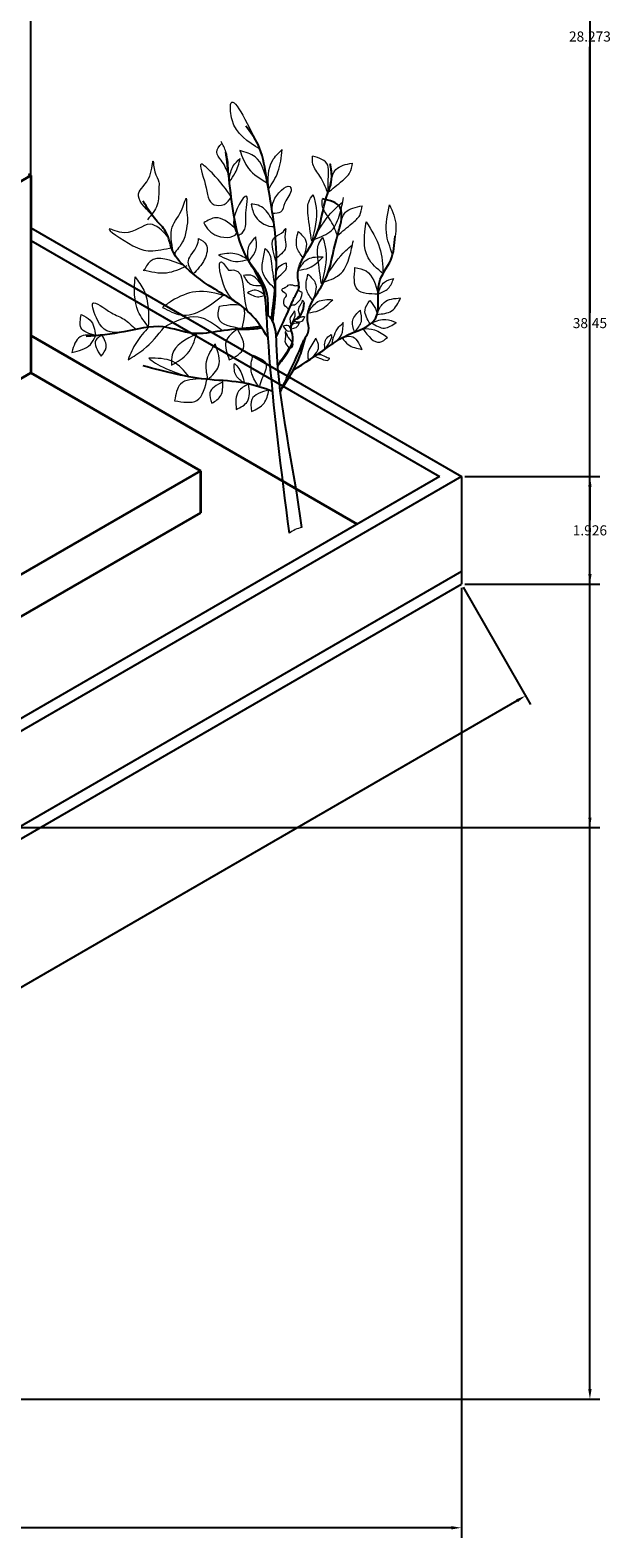
# Model space of a CAD drawing. Units: metres. Extents: x 12735 to 25554, y 20954 to 41989.
# Tile 14 of 15: x 12773 to 12784, y 20954 to 20981. Entities that reach past the tile are written whole.
import ezdxf

# ---------------------------------------------------------------- set-up
doc = ezdxf.new("R2010")
doc.units = ezdxf.units.M
doc.layers.get('Defpoints').update_dxf_attribs({"lineweight": 13})
for name, color, linetype, lineweight in [('A-ANNO-DIMS', 2, 'Continuous', 18), ('A-ELEV', 7, 'Continuous', 35), ('C-SITE', 8, 'Continuous', 25), ('TREES', 72, 'Continuous', 18)]:
    doc.layers.add(name, color=color, linetype=linetype, lineweight=lineweight)
doc.layers.add('STEM', color=32, linetype='Continuous')
doc.styles.get("Standard").update_dxf_attribs({"font": 'arial.ttf'})
doc.dimstyles.get("Standard").update_dxf_attribs({"dimtxt": 0.18, "dimasz": 0.18, "dimexe": 0.18, "dimexo": 0.0625, "dimgap": 0.09, "dimtad": 0, "dimtih": 1, "dimtoh": 1, "dimdec": 4, "dimzin": 0, "dimdsep": 46, "dimtxsty": 'Standard', "dimcen": 0.09, "dimadec": 0, "dimazin": 0, "dimtfac": 1, "dimtdec": 4, "dimtofl": 0, "dimtmove": 0, "dimatfit": 3, "dimfxl": 1, "dimtolj": 1, "dimtzin": 0, "dimarcsym": 0})

# ---------------------------------------------------------------- blocks, each defined once
blk = doc.blocks.new('TREES')
blk.add_line((12743.7, 20972.648), (12743.7, 20972.648))
at = {"layer": 'STEM'}
for points, knots in [([(12743.791, 20972.546), (12743.793, 20972.564), (12743.795, 20972.582), (12743.797, 20972.6), (12743.801, 20972.637), (12743.806, 20972.674), (12743.81, 20972.711), (12743.845, 20973.018), (12743.938, 20973.826), (12743.743, 20974.806), (12743.607, 20975.634), (12743.413, 20975.893), (12743.333, 20975.999)], [-0.164913, -0.164913, -0.164913, -0.164913, -0.110972, -0.110972, -0.110972, 0, 0, 0, 0.920963, 2.426088, 2.990404, 3.384799, 3.384799, 3.384799, 3.384799]), ([(12743.7, 20972.648), (12743.691, 20972.807), (12743.671, 20973.194), (12743.257, 20973.699), (12743.111, 20974.379), (12743.038, 20974.998), (12742.993, 20975.377), (12742.974, 20975.54)], [0, 0, 0, 0, 0.469346, 1.137622, 1.869488, 2.521439, 3.013071, 3.013071, 3.013071, 3.013071]), ([(12743.874, 20972.227), (12743.898, 20972.277), (12743.921, 20972.328), (12743.945, 20972.378), (12744.022, 20972.541), (12744.105, 20972.717), (12744.205, 20972.963), (12744.312, 20973.088), (12744.183, 20973.501), (12744.667, 20973.973), (12744.707, 20974.64), (12744.896, 20975.012), (12744.823, 20975.434), (12744.85, 20975.23), (12744.867, 20975.1)], [-0.166951, -0.166951, -0.166951, -0.166951, 0, 0, 0, 0.539768, 0.582066, 0.798222, 0.98781, 1.7696, 2.524754, 2.899414, 3.105113, 3.460848, 3.460848, 3.460848, 3.460848]), ([(12743.728, 20972.218), (12743.63, 20972.372), (12743.383, 20972.76), (12742.753, 20973.07), (12742.291, 20973.419), (12741.984, 20973.759), (12741.959, 20974.098), (12741.675, 20974.346), (12741.563, 20974.543), (12741.494, 20974.663)], [0, 0, 0, 0, 0.542161, 1.359078, 2.03444, 2.290187, 2.703676, 2.968549, 3.382864, 3.382864, 3.382864, 3.382864]), ([(12743.967, 20971.294), (12743.987, 20971.335), (12744.006, 20971.376), (12744.026, 20971.417), (12744.057, 20971.483), (12744.088, 20971.549), (12744.119, 20971.615), (12744.196, 20971.778), (12744.279, 20971.954), (12744.378, 20972.2), (12744.486, 20972.325), (12744.357, 20972.738), (12744.836, 20973.215), (12744.895, 20973.862), (12745.051, 20974.269), (12745.045, 20974.62), (12744.834, 20974.67), (12744.7, 20974.701)], [-0.355099, -0.355099, -0.355099, -0.355099, -0.218492, -0.218492, -0.218492, 0, 0, 0, 0.539768, 0.582066, 0.798222, 0.98781, 1.7696, 2.524754, 2.899414, 3.105113, 3.460848, 3.460848, 3.460848, 3.460848]), ([(12744.175, 20971.633), (12744.383, 20971.767), (12744.692, 20971.967), (12745.149, 20972.305), (12745.828, 20972.463), (12745.606, 20973.185), (12745.967, 20973.583), (12745.99, 20973.882), (12746.002, 20974.029)], [0, 0, 0, 0, 0.736164, 1.094646, 1.754618, 2.392389, 2.840214, 3.27091, 3.27091, 3.27091, 3.27091]), ([(12743.381, 20973.588), (12743.52, 20973.4), (12743.728, 20973.118), (12743.725, 20972.776), (12743.724, 20972.661), (12743.724, 20972.661), (12743.724, 20972.661), (12743.724, 20972.661), (12743.724, 20972.65), (12743.724, 20972.639), (12743.724, 20972.627)], [0, 0, 0, 0, 0.673099, 1.009429, 1.009429, 1.009429, 1.009429, 1.009429, 1.009429, 1.043412, 1.043412, 1.043412, 1.043412]), ([(12743.814, 20972.505), (12743.817, 20972.531), (12743.819, 20972.556), (12743.822, 20972.581), (12743.827, 20972.63), (12743.832, 20972.679), (12743.838, 20972.727), (12743.847, 20972.813), (12743.865, 20972.982), (12743.864, 20973.152), (12743.864, 20973.236)], [-0.2227932, -0.2227932, -0.2227932, -0.2227932, -0.1464713, -0.1464713, -0.1464713, 0, 0, 0, 0.2578951, 0.5103882, 0.5103882, 0.5103882, 0.5103882]), ([(12743.902, 20971.717), (12743.93, 20971.754), (12743.959, 20971.791), (12743.988, 20971.829), (12743.988, 20971.829), (12743.988, 20971.829), (12743.988, 20971.829), (12744.096, 20971.973), (12744.236, 20972.16), (12744.082, 20972.476), (12744.347, 20972.598), (12744.368, 20972.766), (12744.376, 20972.837)], [-0.129757, -0.129757, -0.129757, -0.129757, 0, 0, 0, 0, 0, 0, 0.485118, 0.62751, 0.913144, 1.120766, 1.120766, 1.120766, 1.120766]), ([(12744.111, 20968.725), (12743.967, 20969.837), (12743.799, 20971.142), (12743.712, 20972.453), (12743.7, 20972.648)], [0, 0, 0, 0, 3.359203, 3.944548, 3.944548, 3.944548, 3.944548]), ([(12744.332, 20968.825), (12744.189, 20969.936), (12743.871, 20971.161), (12743.872, 20972.51), (12743.7, 20972.648)], [0, 0, 0, 0, 3.359203, 3.972384, 3.972384, 3.972384, 3.972384]), ([(12743.597, 20972.418), (12743.533, 20972.41), (12743.292, 20972.379), (12742.889, 20972.351), (12742.364, 20972.241), (12741.803, 20972.489), (12741.157, 20972.302), (12740.698, 20972.258), (12740.474, 20972.237)], [0, 0, 0, 0, 0.193148, 0.727923, 1.218416, 1.762371, 2.471743, 3.152626, 3.152626, 3.152626, 3.152626]), ([(12743.181, 20972.372), (12743.296, 20972.37), (12743.441, 20972.368), (12743.583, 20972.39), (12743.613, 20972.395)], [0, 0, 0, 0, 0.3435042, 0.4329772, 0.4329772, 0.4329772, 0.4329772]), ([(12743.948, 20971.264), (12743.975, 20971.305), (12744.002, 20971.345), (12744.029, 20971.386), (12744.029, 20971.386), (12744.029, 20971.386), (12744.029, 20971.386), (12744.129, 20971.55), (12744.289, 20971.812), (12744.368, 20972.107), (12744.398, 20972.218)], [-0.148605, -0.148605, -0.148605, -0.148605, 0, 0, 0, 0, 0, 0, 0.572176, 0.914425, 0.914425, 0.914425, 0.914425]), ([(12743.901, 20971.729), (12743.929, 20971.768), (12743.958, 20971.808), (12743.986, 20971.847), (12743.986, 20971.847), (12743.986, 20971.847), (12743.986, 20971.847), (12744.02, 20971.892), (12744.062, 20971.951), (12744.099, 20972.014), (12744.107, 20972.028)], [-0.1467707, -0.1467707, -0.1467707, -0.1467707, 0, 0, 0, 0, 0, 0, 0.1684242, 0.2179474, 0.2179474, 0.2179474, 0.2179474]), ([(12743.81, 20971.258), (12743.646, 20971.316), (12743.283, 20971.443), (12742.486, 20971.453), (12741.888, 20971.61), (12741.494, 20971.714)], [0, 0, 0, 0, 0.519056, 1.146346, 2.366016, 2.366016, 2.366016, 2.366016])]:
    blk.add_open_spline(points, degree=3, knots=knots, dxfattribs=at)
blk.add_open_spline([(12744.644, 20971.941), (12744.672, 20971.961), (12744.701, 20971.98), (12744.73, 20972)], degree=3, dxfattribs=at)
at = {"layer": 'TREES'}
for points, knots in [([(12743.584, 20975.586), (12743.37, 20975.718), (12743.075, 20975.9), (12743.022, 20976.725), (12743.333, 20976.097), (12743.574, 20975.612)], [0, 0, 0, 0, 0.724771, 1.002271, 1.932196, 1.932196, 1.932196, 1.932196]), ([(12743.021, 20975.14), (12742.985, 20975.224), (12742.928, 20975.356), (12742.766, 20975.539), (12742.854, 20975.638), (12742.901, 20975.69)], [0, 0, 0, 0, 0.2845416, 0.4465287, 0.6279758, 0.6279758, 0.6279758, 0.6279758]), ([(12743.021, 20975.14), (12743.019, 20975.277), (12743.016, 20975.483), (12742.921, 20975.662), (12742.889, 20975.721)], [0, 0, 0, 0, 0.4023849, 0.6031293, 0.6031293, 0.6031293, 0.6031293]), ([(12743.031, 20975.058), (12743.048, 20975.139), (12743.077, 20975.281), (12743.184, 20975.377), (12743.231, 20975.418)], [0, 0, 0, 0, 0.2398723, 0.4207027, 0.4207027, 0.4207027, 0.4207027]), ([(12743.037, 20975.007), (12743.075, 20975.058), (12743.166, 20975.181), (12743.207, 20975.33), (12743.231, 20975.418)], [0, 0, 0, 0, 0.1895117, 0.457602, 0.457602, 0.457602, 0.457602]), ([(12743.718, 20974.979), (12743.671, 20975.164), (12743.598, 20975.454), (12743.323, 20975.534), (12743.223, 20975.563)], [0, 0, 0, 0, 0.519429, 0.8155501, 0.8155501, 0.8155501, 0.8155501]), ([(12743.223, 20975.563), (12743.266, 20975.448), (12743.36, 20975.195), (12743.592, 20975.055), (12743.718, 20974.979)], [0, 0, 0, 0, 0.3595778, 0.7860105, 0.7860105, 0.7860105, 0.7860105]), ([(12743.737, 20974.871), (12743.729, 20975.055), (12743.718, 20975.333), (12743.914, 20975.516), (12743.981, 20975.578)], [0, 0, 0, 0, 0.5134638, 0.7779111, 0.7779111, 0.7779111, 0.7779111]), ([(12743.737, 20974.871), (12743.801, 20974.971), (12743.939, 20975.186), (12743.966, 20975.441), (12743.981, 20975.578)], [0, 0, 0, 0, 0.351068, 0.7565079, 0.7565079, 0.7565079, 0.7565079]), ([(12744.796, 20974.806), (12744.757, 20974.909), (12744.688, 20975.088), (12744.514, 20975.28), (12744.523, 20975.414), (12744.526, 20975.464)], [0, 0, 0, 0, 0.3323117, 0.5782809, 0.7232611, 0.7232611, 0.7232611, 0.7232611]), ([(12744.805, 20974.813), (12744.804, 20974.918), (12744.803, 20975.076), (12744.822, 20975.37), (12744.643, 20975.427), (12744.526, 20975.464)], [0, 0, 0, 0, 0.3224266, 0.4885617, 0.8037384, 0.8037384, 0.8037384, 0.8037384]), ([(12741.648, 20974.411), (12741.519, 20974.547), (12741.281, 20974.798), (12741.642, 20974.995), (12741.673, 20975.511), (12741.684, 20975.149), (12741.787, 20975.033), (12741.768, 20974.824), (12741.781, 20974.575), (12741.641, 20974.411), (12741.569, 20974.326)], [0, 0, 0, 0, 0.446457, 0.821839, 1.096823, 1.294203, 1.491123, 1.594729, 1.894892, 2.216107, 2.216107, 2.216107, 2.216107]), ([(12743.07, 20974.733), (12742.98, 20974.863), (12742.848, 20975.053), (12742.433, 20975.446), (12742.649, 20974.915), (12742.651, 20974.573), (12742.961, 20974.576), (12743.034, 20974.678), (12743.071, 20974.73)], [0, 0, 0, 0, 0.54832, 0.799685, 1.166614, 1.565159, 1.742127, 1.925713, 1.925713, 1.925713, 1.925713]), ([(12744.796, 20974.806), (12744.882, 20974.878), (12745.017, 20974.992), (12745.211, 20975.15), (12745.228, 20975.277), (12745.236, 20975.337)], [0, 0, 0, 0, 0.3416822, 0.5370609, 0.7122352, 0.7122352, 0.7122352, 0.7122352]), ([(12744.839, 20974.951), (12744.859, 20975.055), (12744.903, 20975.272), (12745.122, 20975.315), (12745.236, 20975.337)], [0, 0, 0, 0, 0.2913456, 0.6064398, 0.6064398, 0.6064398, 0.6064398]), ([(12743.814, 20974.4), (12743.798, 20974.494), (12743.764, 20974.693), (12744.115, 20975.006), (12744.156, 20974.79), (12744.01, 20974.677), (12743.989, 20974.434), (12743.864, 20974.438), (12743.809, 20974.439)], [0, 0, 0, 0, 0.311146, 0.650746, 0.669061, 0.940573, 1.125337, 1.270427, 1.270427, 1.270427, 1.270427]), ([(12742.028, 20973.754), (12742.003, 20973.912), (12741.953, 20974.218), (12742.174, 20974.414), (12742.283, 20974.81), (12742.258, 20974.48), (12742.304, 20974.323), (12742.246, 20974.069), (12742.227, 20973.932), (12742.006, 20973.671), (12742.066, 20973.72), (12742.075, 20973.727)], [0, 0, 0, 0, 0.436736, 0.842969, 1.012738, 1.21393, 1.403734, 1.613178, 1.897283, 2.067562, 2.097274, 2.097274, 2.097274, 2.097274]), ([(12743.191, 20974.047), (12743.14, 20974.139), (12743.026, 20974.346), (12743.367, 20974.877), (12743.354, 20974.597), (12743.309, 20974.413), (12743.358, 20974.125), (12743.218, 20974.059), (12743.191, 20974.047)], [0, 0, 0, 0, 0.337622, 0.758697, 0.837919, 1.040495, 1.406258, 1.489574, 1.489574, 1.489574, 1.489574]), ([(12744.509, 20973.941), (12744.486, 20974.093), (12744.451, 20974.322), (12744.425, 20974.623), (12744.504, 20974.731), (12744.534, 20974.773)], [0, 0, 0, 0, 0.4681587, 0.7056034, 0.8580265, 0.8580265, 0.8580265, 0.8580265]), ([(12744.534, 20974.773), (12744.556, 20974.698), (12744.634, 20974.425), (12744.562, 20974.144), (12744.509, 20973.941)], [0, 0, 0, 0, 0.2327329, 0.8431329, 0.8431329, 0.8431329, 0.8431329]), ([(12744.554, 20973.975), (12744.669, 20974.016), (12744.893, 20974.094), (12745.019, 20974.421), (12745.06, 20974.624), (12745.08, 20974.72)], [0, 0, 0, 0, 0.348929, 0.678298, 0.9763146, 0.9763146, 0.9763146, 0.9763146]), ([(12744.618, 20974.118), (12744.717, 20974.268), (12744.844, 20974.462), (12745.022, 20974.606), (12745.062, 20974.638)], [0, 0, 0, 0, 0.5333846, 0.686651, 0.686651, 0.686651, 0.686651]), ([(12744.97, 20974.043), (12744.931, 20974.146), (12744.862, 20974.325), (12744.688, 20974.517), (12744.697, 20974.651), (12744.7, 20974.701)], [0, 0, 0, 0, 0.3323117, 0.5782809, 0.7232611, 0.7232611, 0.7232611, 0.7232611]), ([(12743.128, 20974.182), (12743.019, 20974.275), (12742.841, 20974.427), (12742.65, 20974.313), (12742.577, 20974.27)], [0, 0, 0, 0, 0.3785086, 0.6144536, 0.6144536, 0.6144536, 0.6144536]), ([(12743.835, 20974.249), (12743.789, 20974.346), (12743.724, 20974.484), (12743.556, 20974.594), (12743.468, 20974.601), (12743.424, 20974.604)], [0, 0, 0, 0, 0.3158223, 0.4463774, 0.5774617, 0.5774617, 0.5774617, 0.5774617]), ([(12743.424, 20974.604), (12743.442, 20974.527), (12743.487, 20974.324), (12743.715, 20974.191), (12743.841, 20974.206), (12743.841, 20974.206)], [0, 0, 0, 0, 0.2361186, 0.6165307, 0.6167763, 0.6167763, 0.6167763, 0.6167763]), ([(12744.97, 20974.043), (12745.056, 20974.115), (12745.191, 20974.229), (12745.385, 20974.387), (12745.402, 20974.514), (12745.41, 20974.574)], [0, 0, 0, 0, 0.3416822, 0.5370609, 0.7122352, 0.7122352, 0.7122352, 0.7122352]), ([(12745.013, 20974.188), (12745.033, 20974.292), (12745.077, 20974.509), (12745.296, 20974.552), (12745.41, 20974.574)], [0, 0, 0, 0, 0.2913456, 0.6064398, 0.6064398, 0.6064398, 0.6064398]), ([(12745.957, 20973.706), (12745.908, 20973.835), (12745.798, 20974.123), (12745.864, 20974.427), (12745.9, 20974.594)], [0, 0, 0, 0, 0.4051126, 0.906838, 0.906838, 0.906838, 0.906838]), ([(12745.9, 20974.594), (12745.955, 20974.471), (12746.037, 20974.287), (12746.01, 20974.092), (12746.002, 20974.029)], [0, 0, 0, 0, 0.3943838, 0.5836156, 0.5836156, 0.5836156, 0.5836156]), ([(12741.943, 20974.016), (12741.835, 20974.13), (12741.594, 20974.382), (12741.272, 20973.991), (12740.687, 20974.27), (12741.289, 20973.836), (12741.63, 20973.742), (12741.878, 20973.799), (12742.016, 20973.831)], [0, 0, 0, 0, 0.397812, 0.88569, 1.156328, 1.66735, 1.991498, 2.394837, 2.394837, 2.394837, 2.394837]), ([(12742.577, 20974.27), (12742.635, 20974.174), (12742.755, 20973.977), (12743.187, 20974.003), (12743.173, 20974.131), (12743.172, 20974.137)], [0, 0, 0, 0, 0.3386751, 0.6999446, 0.7185805, 0.7185805, 0.7185805, 0.7185805]), ([(12743.879, 20973.555), (12743.816, 20973.752), (12743.731, 20974.021), (12743.982, 20974.067), (12744.068, 20974.224), (12744.006, 20973.984), (12744.093, 20973.824), (12743.961, 20973.709), (12743.879, 20973.638)], [0, 0, 0, 0, 0.469961, 0.638827, 0.705595, 0.853148, 1.022788, 1.296962, 1.296962, 1.296962, 1.296962]), ([(12744.356, 20973.647), (12744.309, 20973.708), (12744.202, 20973.846), (12744.245, 20974.018), (12744.268, 20974.113)], [0, 0, 0, 0, 0.2209277, 0.4981889, 0.4981889, 0.4981889, 0.4981889]), ([(12744.268, 20974.113), (12744.323, 20974.065), (12744.46, 20973.94), (12744.395, 20973.758), (12744.356, 20973.647)], [0, 0, 0, 0, 0.203616, 0.5174389, 0.5174389, 0.5174389, 0.5174389]), ([(12745.785, 20973.361), (12745.68, 20973.449), (12745.404, 20973.684), (12745.451, 20974.057), (12745.481, 20974.288)], [0, 0, 0, 0, 0.391493, 1.034106, 1.034106, 1.034106, 1.034106]), ([(12745.481, 20974.288), (12745.577, 20974.138), (12745.76, 20973.855), (12745.777, 20973.519), (12745.785, 20973.361)], [0, 0, 0, 0, 0.5245256, 0.9915723, 0.9915723, 0.9915723, 0.9915723]), ([(12742.389, 20973.356), (12742.341, 20973.437), (12742.234, 20973.617), (12742.458, 20973.799), (12742.48, 20973.946), (12742.486, 20973.991)], [0, 0, 0, 0, 0.251735, 0.5591808, 0.6938707, 0.6938707, 0.6938707, 0.6938707]), ([(12742.486, 20973.991), (12742.542, 20973.959), (12742.68, 20973.88), (12742.598, 20973.572), (12742.464, 20973.433), (12742.389, 20973.356)], [0, 0, 0, 0, 0.1746142, 0.4385715, 0.7703441, 0.7703441, 0.7703441, 0.7703441]), ([(12743.381, 20973.588), (12743.369, 20973.67), (12743.344, 20973.833), (12743.453, 20973.958), (12743.508, 20974.02)], [0, 0, 0, 0, 0.2360196, 0.4713289, 0.4713289, 0.4713289, 0.4713289]), ([(12743.381, 20973.588), (12743.434, 20973.649), (12743.541, 20973.774), (12743.519, 20973.937), (12743.508, 20974.02)], [0, 0, 0, 0, 0.2309694, 0.4699481, 0.4699481, 0.4699481, 0.4699481]), ([(12743.851, 20973.09), (12743.747, 20973.196), (12743.578, 20973.368), (12743.647, 20973.644), (12743.671, 20973.769), (12743.679, 20973.81)], [0, 0, 0, 0, 0.4076044, 0.6640272, 0.7921335, 0.7921335, 0.7921335, 0.7921335]), ([(12743.679, 20973.81), (12743.708, 20973.778), (12743.776, 20973.703), (12743.798, 20973.443), (12743.829, 20973.238), (12743.851, 20973.09)], [0, 0, 0, 0, 0.125659, 0.2981213, 0.7527794, 0.7527794, 0.7527794, 0.7527794]), ([(12744.683, 20973.178), (12744.66, 20973.33), (12744.625, 20973.559), (12744.599, 20973.86), (12744.677, 20973.968), (12744.708, 20974.01)], [0, 0, 0, 0, 0.4681587, 0.7056034, 0.8580265, 0.8580265, 0.8580265, 0.8580265]), ([(12744.708, 20974.01), (12744.73, 20973.935), (12744.807, 20973.662), (12744.735, 20973.381), (12744.683, 20973.178)], [0, 0, 0, 0, 0.2327329, 0.8431329, 0.8431329, 0.8431329, 0.8431329]), ([(12744.728, 20973.213), (12744.843, 20973.253), (12745.067, 20973.331), (12745.193, 20973.658), (12745.234, 20973.861), (12745.254, 20973.957)], [0, 0, 0, 0, 0.348929, 0.678298, 0.9763146, 0.9763146, 0.9763146, 0.9763146]), ([(12744.792, 20973.355), (12744.891, 20973.505), (12745.018, 20973.699), (12745.196, 20973.843), (12745.236, 20973.876)], [0, 0, 0, 0, 0.5333846, 0.686651, 0.686651, 0.686651, 0.686651]), ([(12742.221, 20973.506), (12741.989, 20973.602), (12741.674, 20973.731), (12741.536, 20973.471), (12741.5, 20973.404)], [0, 0, 0, 0, 0.6060397, 0.8197481, 0.8197481, 0.8197481, 0.8197481]), ([(12743.253, 20972.784), (12743.147, 20972.854), (12742.919, 20973.005), (12742.8, 20973.728), (12742.973, 20973.491), (12743.022, 20973.422)], [0, 0, 0, 0, 0.420416, 0.90702, 1.103207, 1.103207, 1.103207, 1.103207]), ([(12743.364, 20973.617), (12743.288, 20973.661), (12743.124, 20973.754), (12742.939, 20973.715), (12742.84, 20973.694)], [0, 0, 0, 0, 0.2535199, 0.5460217, 0.5460217, 0.5460217, 0.5460217]), ([(12742.84, 20973.694), (12742.956, 20973.634), (12743.128, 20973.545), (12743.306, 20973.6), (12743.364, 20973.617)], [0, 0, 0, 0, 0.369417, 0.546183, 0.546183, 0.546183, 0.546183]), ([(12743.864, 20973.236), (12743.891, 20973.272), (12743.952, 20973.35), (12744.077, 20973.438), (12744.058, 20973.527), (12744.051, 20973.558)], [0, 0, 0, 0, 0.1377377, 0.3031534, 0.3935537, 0.3935537, 0.3935537, 0.3935537]), ([(12743.866, 20973.267), (12743.872, 20973.352), (12743.881, 20973.49), (12744.004, 20973.539), (12744.051, 20973.558)], [0, 0, 0, 0, 0.2295676, 0.3730638, 0.3730638, 0.3730638, 0.3730638]), ([(12744.268, 20973.425), (12744.32, 20973.505), (12744.424, 20973.666), (12744.615, 20973.662), (12744.711, 20973.66)], [0, 0, 0, 0, 0.2669279, 0.5349854, 0.5349854, 0.5349854, 0.5349854]), ([(12744.268, 20973.425), (12744.336, 20973.433), (12744.51, 20973.454), (12744.635, 20973.582), (12744.711, 20973.66)], [0, 0, 0, 0, 0.1990667, 0.5143408, 0.5143408, 0.5143408, 0.5143408]), ([(12741.595, 20972.406), (12741.523, 20972.496), (12741.318, 20972.752), (12741.336, 20973.087), (12741.348, 20973.304)], [0, 0, 0, 0, 0.3390919, 0.9589007, 0.9589007, 0.9589007, 0.9589007]), ([(12741.348, 20973.304), (12741.406, 20973.227), (12741.6, 20972.969), (12741.591, 20972.637), (12741.585, 20972.405)], [0, 0, 0, 0, 0.2865181, 0.9509807, 0.9509807, 0.9509807, 0.9509807]), ([(12741.493, 20973.429), (12741.634, 20973.396), (12741.906, 20973.333), (12742.16, 20973.449), (12742.283, 20973.505)], [0, 0, 0, 0, 0.420024, 0.8136231, 0.8136231, 0.8136231, 0.8136231]), ([(12743.022, 20973.422), (12743.059, 20973.426), (12743.334, 20973.456), (12743.256, 20972.956), (12743.349, 20972.723), (12743.36, 20972.696)], [0, 0, 0, 0, 0.1039343, 0.7792863, 0.8705393, 0.8705393, 0.8705393, 0.8705393]), ([(12743.621, 20973.151), (12743.561, 20973.233), (12743.473, 20973.354), (12743.333, 20973.334), (12743.288, 20973.327)], [0, 0, 0, 0, 0.2726158, 0.4022356, 0.4022356, 0.4022356, 0.4022356]), ([(12743.288, 20973.327), (12743.325, 20973.265), (12743.399, 20973.138), (12743.546, 20973.147), (12743.621, 20973.151)], [0, 0, 0, 0, 0.199886, 0.4070645, 0.4070645, 0.4070645, 0.4070645]), ([(12744.53, 20972.884), (12744.482, 20972.945), (12744.376, 20973.084), (12744.419, 20973.255), (12744.442, 20973.351)], [0, 0, 0, 0, 0.2209277, 0.4981889, 0.4981889, 0.4981889, 0.4981889]), ([(12744.442, 20973.351), (12744.496, 20973.302), (12744.634, 20973.177), (12744.569, 20972.995), (12744.53, 20972.884)], [0, 0, 0, 0, 0.203616, 0.5174389, 0.5174389, 0.5174389, 0.5174389]), ([(12745.697, 20972.996), (12745.547, 20972.999), (12745.238, 20973.004), (12745.268, 20973.314), (12745.283, 20973.473)], [0, 0, 0, 0, 0.3799868, 0.779071, 0.779071, 0.779071, 0.779071]), ([(12745.283, 20973.473), (12745.354, 20973.458), (12745.585, 20973.409), (12745.651, 20973.165), (12745.697, 20972.996)], [0, 0, 0, 0, 0.2074949, 0.6743984, 0.6743984, 0.6743984, 0.6743984]), ([(12745.697, 20972.996), (12745.724, 20973.08), (12745.77, 20973.226), (12745.915, 20973.262), (12745.976, 20973.277)], [0, 0, 0, 0, 0.2439478, 0.4222058, 0.4222058, 0.4222058, 0.4222058]), ([(12745.697, 20972.996), (12745.764, 20973.024), (12745.897, 20973.078), (12745.95, 20973.211), (12745.976, 20973.277)], [0, 0, 0, 0, 0.2073861, 0.4117039, 0.4117039, 0.4117039, 0.4117039]), ([(12742.983, 20972.961), (12742.799, 20973.009), (12742.463, 20973.098), (12742.071, 20972.928), (12741.893, 20972.798), (12741.839, 20972.759)], [0, 0, 0, 0, 0.553894, 1.01265, 1.215779, 1.215779, 1.215779, 1.215779]), ([(12743.669, 20972.977), (12743.606, 20973.025), (12743.504, 20973.102), (12743.398, 20973.043), (12743.358, 20973.021)], [0, 0, 0, 0, 0.2119595, 0.340544, 0.340544, 0.340544, 0.340544]), ([(12743.358, 20973.021), (12743.426, 20972.983), (12743.527, 20972.926), (12743.633, 20972.964), (12743.669, 20972.977)], [0, 0, 0, 0, 0.2166399, 0.3265492, 0.3265492, 0.3265492, 0.3265492]), ([(12744.074, 20972.655), (12744.086, 20972.673), (12744.124, 20972.731), (12743.998, 20972.782), (12744.014, 20972.867), (12744.011, 20972.925), (12744.052, 20972.944), (12744.07, 20973.015), (12743.988, 20973.027), (12743.97, 20973.091), (12744.03, 20973.11), (12744.072, 20973.132), (12744.097, 20973.169), (12744.133, 20973.163), (12744.172, 20973.164), (12744.216, 20973.136), (12744.296, 20973.17), (12744.282, 20973.105), (12744.259, 20973.057), (12744.341, 20973.048), (12744.328, 20972.986), (12744.32, 20972.935), (12744.299, 20972.884), (12744.258, 20972.852), (12744.236, 20972.821), (12744.215, 20972.805), (12744.179, 20972.793), (12744.139, 20972.807), (12744.095, 20972.746), (12744.111, 20972.739), (12744.111, 20972.739)], [0, 0, 0, 0, 0.055886, 0.185472, 0.25227, 0.305988, 0.338368, 0.378405, 0.48523, 0.4997, 0.565031, 0.618654, 0.656012, 0.680602, 0.71942, 0.77395, 0.836088, 0.890088, 0.913694, 0.979696, 1.032481, 1.0683, 1.142133, 1.186825, 1.224162, 1.25438, 1.26551, 1.333296, 1.383591, 1.385324, 1.385324, 1.385324, 1.385324]), ([(12741.358, 20972.366), (12741.291, 20972.434), (12741.162, 20972.564), (12740.909, 20972.646), (12740.492, 20972.989), (12740.719, 20972.381), (12740.905, 20972.253), (12741.437, 20972.382), (12741.361, 20972.366), (12741.358, 20972.366)], [0, 0, 0, 0, 0.274554, 0.529523, 0.902439, 1.220606, 1.740632, 1.953969, 1.962894, 1.962894, 1.962894, 1.962894]), ([(12741.839, 20972.759), (12741.949, 20972.7), (12742.323, 20972.501), (12742.684, 20972.786), (12742.939, 20972.987)], [0, 0, 0, 0, 0.355589, 1.206871, 1.206871, 1.206871, 1.206871]), ([(12743.257, 20972.379), (12743.071, 20972.409), (12742.794, 20972.453), (12742.842, 20972.698), (12742.858, 20972.779)], [0, 0, 0, 0, 0.4478858, 0.6692237, 0.6692237, 0.6692237, 0.6692237]), ([(12742.858, 20972.779), (12743.034, 20972.81), (12743.375, 20972.87), (12743.295, 20972.539), (12743.257, 20972.379)], [0, 0, 0, 0, 0.4156133, 0.8046117, 0.8046117, 0.8046117, 0.8046117]), ([(12744.299, 20972.615), (12744.284, 20972.657), (12744.255, 20972.734), (12744.322, 20972.816), (12744.34, 20972.869), (12744.347, 20972.89)], [0, 0, 0, 0, 0.1248577, 0.2264879, 0.2926557, 0.2926557, 0.2926557, 0.2926557]), ([(12744.442, 20972.662), (12744.494, 20972.743), (12744.598, 20972.903), (12744.789, 20972.899), (12744.885, 20972.897)], [0, 0, 0, 0, 0.2669279, 0.5349854, 0.5349854, 0.5349854, 0.5349854]), ([(12744.442, 20972.662), (12744.51, 20972.671), (12744.684, 20972.691), (12744.809, 20972.819), (12744.885, 20972.897)], [0, 0, 0, 0, 0.1990667, 0.5143408, 0.5143408, 0.5143408, 0.5143408]), ([(12745.557, 20972.46), (12745.505, 20972.545), (12745.415, 20972.69), (12745.509, 20972.826), (12745.548, 20972.882)], [0, 0, 0, 0, 0.2672291, 0.4594629, 0.4594629, 0.4594629, 0.4594629]), ([(12745.548, 20972.882), (12745.623, 20972.785), (12745.735, 20972.639), (12745.619, 20972.519), (12745.581, 20972.479)], [0, 0, 0, 0, 0.3063433, 0.4579535, 0.4579535, 0.4579535, 0.4579535]), ([(12745.681, 20972.634), (12745.776, 20972.643), (12745.97, 20972.661), (12746.056, 20972.838), (12746.1, 20972.929)], [0, 0, 0, 0, 0.2646598, 0.5464061, 0.5464061, 0.5464061, 0.5464061]), ([(12745.691, 20972.679), (12745.723, 20972.743), (12745.803, 20972.904), (12745.989, 20972.919), (12746.1, 20972.929)], [0, 0, 0, 0, 0.2025395, 0.5100625, 0.5100625, 0.5100625, 0.5100625]), ([(12740.645, 20972.254), (12740.532, 20972.287), (12740.33, 20972.345), (12740.37, 20972.543), (12740.387, 20972.63)], [0, 0, 0, 0, 0.300298, 0.5327787, 0.5327787, 0.5327787, 0.5327787]), ([(12740.387, 20972.63), (12740.446, 20972.602), (12740.598, 20972.53), (12740.627, 20972.359), (12740.645, 20972.254)], [0, 0, 0, 0, 0.1847401, 0.4807235, 0.4807235, 0.4807235, 0.4807235]), ([(12742.916, 20972.343), (12742.772, 20972.452), (12742.448, 20972.697), (12742.076, 20972.511), (12741.869, 20972.407)], [0, 0, 0, 0, 0.501704, 1.133573, 1.133573, 1.133573, 1.133573]), ([(12744.14, 20972.455), (12744.129, 20972.498), (12744.112, 20972.571), (12744.173, 20972.643), (12744.195, 20972.684), (12744.204, 20972.7)], [0, 0, 0, 0, 0.124617, 0.2107396, 0.2658134, 0.2658134, 0.2658134, 0.2658134]), ([(12744.137, 20972.378), (12744.147, 20972.414), (12744.168, 20972.49), (12744.249, 20972.485), (12744.292, 20972.483)], [0, 0, 0, 0, 0.0982704, 0.2114853, 0.2114853, 0.2114853, 0.2114853]), ([(12744.137, 20972.378), (12744.171, 20972.382), (12744.241, 20972.388), (12744.274, 20972.45), (12744.292, 20972.483)], [0, 0, 0, 0, 0.0955829, 0.1975677, 0.1975677, 0.1975677, 0.1975677]), ([(12744.14, 20972.455), (12744.155, 20972.485), (12744.181, 20972.535), (12744.225, 20972.615), (12744.212, 20972.669), (12744.204, 20972.7)], [0, 0, 0, 0, 0.1037237, 0.1704768, 0.2630686, 0.2630686, 0.2630686, 0.2630686]), ([(12744.192, 20972.515), (12744.244, 20972.502), (12744.335, 20972.479), (12744.372, 20972.56), (12744.387, 20972.593)], [0, 0, 0, 0, 0.1401829, 0.239855, 0.239855, 0.239855, 0.239855]), ([(12744.25, 20972.55), (12744.272, 20972.566), (12744.314, 20972.595), (12744.364, 20972.594), (12744.387, 20972.593)], [0, 0, 0, 0, 0.0790636, 0.1468534, 0.1468534, 0.1468534, 0.1468534]), ([(12744.868, 20972.097), (12744.937, 20972.148), (12745.072, 20972.246), (12745.072, 20972.413), (12745.073, 20972.494)], [0, 0, 0, 0, 0.2403434, 0.4714363, 0.4714363, 0.4714363, 0.4714363]), ([(12744.868, 20972.097), (12744.895, 20972.212), (12744.931, 20972.363), (12745.046, 20972.458), (12745.074, 20972.481)], [0, 0, 0, 0, 0.3374321, 0.4432568, 0.4432568, 0.4432568, 0.4432568]), ([(12745.276, 20972.317), (12745.252, 20972.391), (12745.204, 20972.544), (12745.32, 20972.655), (12745.379, 20972.712)], [0, 0, 0, 0, 0.2148949, 0.4418034, 0.4418034, 0.4418034, 0.4418034]), ([(12745.276, 20972.317), (12745.329, 20972.378), (12745.429, 20972.493), (12745.395, 20972.642), (12745.379, 20972.712)], [0, 0, 0, 0, 0.2259484, 0.4304915, 0.4304915, 0.4304915, 0.4304915]), ([(12745.582, 20972.481), (12745.667, 20972.516), (12745.814, 20972.576), (12745.958, 20972.516), (12746.019, 20972.491)], [0, 0, 0, 0, 0.2625898, 0.453199, 0.453199, 0.453199, 0.453199]), ([(12745.582, 20972.481), (12745.658, 20972.433), (12745.808, 20972.341), (12745.95, 20972.442), (12746.019, 20972.491)], [0, 0, 0, 0, 0.2451587, 0.4783488, 0.4783488, 0.4783488, 0.4783488]), ([(12740.645, 20972.254), (12740.54, 20972.264), (12740.318, 20972.286), (12740.252, 20972.07), (12740.216, 20971.955)], [0, 0, 0, 0, 0.2808571, 0.5946199, 0.5946199, 0.5946199, 0.5946199]), ([(12740.216, 20971.955), (12740.344, 20971.984), (12740.536, 20972.026), (12740.618, 20972.197), (12740.645, 20972.254)], [0, 0, 0, 0, 0.3624795, 0.5464116, 0.5464116, 0.5464116, 0.5464116]), ([(12740.757, 20972.265), (12740.712, 20972.237), (12740.573, 20972.15), (12740.673, 20971.993), (12740.741, 20971.887)], [0, 0, 0, 0, 0.1417373, 0.4445248, 0.4445248, 0.4445248, 0.4445248]), ([(12740.741, 20971.887), (12740.783, 20971.937), (12740.878, 20972.054), (12740.801, 20972.189), (12740.757, 20972.265)], [0, 0, 0, 0, 0.1798963, 0.4162104, 0.4162104, 0.4162104, 0.4162104]), ([(12741.223, 20971.823), (12741.319, 20971.881), (12741.571, 20972.033), (12741.755, 20972.264), (12741.869, 20972.407)], [0, 0, 0, 0, 0.3340001, 0.876507, 0.876507, 0.876507, 0.876507]), ([(12741.595, 20972.406), (12741.515, 20972.319), (12741.356, 20972.147), (12741.267, 20971.93), (12741.223, 20971.823)], [0, 0, 0, 0, 0.3521388, 0.6963584, 0.6963584, 0.6963584, 0.6963584]), ([(12742.453, 20972.29), (12742.257, 20972.189), (12741.999, 20972.056), (12742.001, 20971.792), (12742.002, 20971.729)], [0, 0, 0, 0, 0.5792647, 0.7616052, 0.7616052, 0.7616052, 0.7616052]), ([(12742.002, 20971.729), (12742.108, 20971.788), (12742.333, 20971.914), (12742.411, 20972.161), (12742.453, 20972.29)], [0, 0, 0, 0, 0.3533474, 0.7448355, 0.7448355, 0.7448355, 0.7448355]), ([(12743.181, 20972.372), (12743.094, 20972.305), (12742.907, 20972.162), (12742.991, 20971.938), (12743.035, 20971.819)], [0, 0, 0, 0, 0.2977969, 0.6372286, 0.6372286, 0.6372286, 0.6372286]), ([(12743.035, 20971.819), (12743.147, 20971.88), (12743.383, 20972.009), (12743.25, 20972.247), (12743.181, 20972.372)], [0, 0, 0, 0, 0.3275492, 0.688496, 0.688496, 0.688496, 0.688496]), ([(12744.145, 20972.348), (12744.132, 20972.384), (12744.105, 20972.455), (12744.032, 20972.434), (12743.996, 20972.423)], [0, 0, 0, 0, 0.098996, 0.196743, 0.196743, 0.196743, 0.196743]), ([(12743.996, 20972.423), (12744.027, 20972.377), (12744.069, 20972.315), (12744.13, 20972.341), (12744.146, 20972.347)], [0, 0, 0, 0, 0.1368513, 0.185287, 0.185287, 0.185287, 0.185287]), ([(12744.116, 20972.018), (12744.075, 20972.065), (12744.007, 20972.143), (12744.05, 20972.231), (12744.028, 20972.351), (12744.072, 20972.271), (12744.09, 20972.201), (12744.221, 20972.106), (12744.146, 20972.042), (12744.116, 20972.018)], [0, 0, 0, 0, 0.1633748, 0.2727914, 0.3326965, 0.376171, 0.4524353, 0.6040881, 0.701786, 0.701786, 0.701786, 0.701786]), ([(12744.455, 20971.815), (12744.445, 20971.868), (12744.427, 20971.97), (12744.523, 20972.088), (12744.564, 20972.169), (12744.585, 20972.208)], [0, 0, 0, 0, 0.1538132, 0.2966411, 0.4292928, 0.4292928, 0.4292928, 0.4292928]), ([(12744.455, 20971.815), (12744.544, 20971.891), (12744.679, 20972.008), (12744.609, 20972.157), (12744.585, 20972.208)], [0, 0, 0, 0, 0.3019229, 0.4589929, 0.4589929, 0.4589929, 0.4589929]), ([(12744.746, 20972.012), (12744.742, 20972.047), (12744.733, 20972.118), (12744.771, 20972.218), (12744.826, 20972.252), (12744.849, 20972.268)], [0, 0, 0, 0, 0.1066556, 0.2131282, 0.2966333, 0.2966333, 0.2966333, 0.2966333]), ([(12744.746, 20972.012), (12744.773, 20972.045), (12744.822, 20972.105), (12744.891, 20972.268), (12744.848, 20972.268), (12744.847, 20972.268)], [0, 0, 0, 0, 0.1585708, 0.2833525, 0.285588, 0.285588, 0.285588, 0.285588]), ([(12745.053, 20972.215), (12745.111, 20972.233), (12745.273, 20972.284), (12745.353, 20972.117), (12745.405, 20972.009)], [0, 0, 0, 0, 0.1646898, 0.4645687, 0.4645687, 0.4645687, 0.4645687]), ([(12745.053, 20972.215), (12745.087, 20972.171), (12745.174, 20972.057), (12745.317, 20972.027), (12745.405, 20972.009)], [0, 0, 0, 0, 0.1638697, 0.4194041, 0.4194041, 0.4194041, 0.4194041]), ([(12745.422, 20972.381), (12745.493, 20972.379), (12745.657, 20972.373), (12745.791, 20972.276), (12745.866, 20972.222)], [0, 0, 0, 0, 0.2087211, 0.4811791, 0.4811791, 0.4811791, 0.4811791]), ([(12745.422, 20972.381), (12745.521, 20972.247), (12745.661, 20972.058), (12745.82, 20972.185), (12745.866, 20972.222)], [0, 0, 0, 0, 0.3912381, 0.5526272, 0.5526272, 0.5526272, 0.5526272]), ([(12742.652, 20971.471), (12742.63, 20971.58), (12742.585, 20971.809), (12742.714, 20972.005), (12742.781, 20972.107)], [0, 0, 0, 0, 0.3207709, 0.6721329, 0.6721329, 0.6721329, 0.6721329]), ([(12742.652, 20971.471), (12742.732, 20971.545), (12742.92, 20971.718), (12742.832, 20971.965), (12742.781, 20972.107)], [0, 0, 0, 0, 0.3028446, 0.7080533, 0.7080533, 0.7080533, 0.7080533]), ([(12744.561, 20971.885), (12744.589, 20971.902), (12744.651, 20971.938), (12744.742, 20971.883), (12744.801, 20971.859), (12744.827, 20971.849)], [0, 0, 0, 0, 0.0920276, 0.2010844, 0.2860976, 0.2860976, 0.2860976, 0.2860976]), ([(12742.314, 20971.521), (12742.225, 20971.627), (12742.039, 20971.851), (12741.746, 20971.851), (12741.593, 20971.851)], [0, 0, 0, 0, 0.3968877, 0.8302181, 0.8302181, 0.8302181, 0.8302181]), ([(12741.593, 20971.851), (12741.666, 20971.793), (12741.821, 20971.668), (12742.447, 20971.471), (12742.312, 20971.521), (12742.311, 20971.521)], [0, 0, 0, 0, 0.3696351, 0.7965164, 0.7990281, 0.7990281, 0.7990281, 0.7990281]), ([(12743.304, 20971.408), (12743.247, 20971.446), (12743.157, 20971.505), (12743.12, 20971.647), (12743.123, 20971.722), (12743.125, 20971.759)], [0, 0, 0, 0, 0.196607, 0.3084716, 0.4203856, 0.4203856, 0.4203856, 0.4203856]), ([(12743.125, 20971.759), (12743.154, 20971.73), (12743.251, 20971.635), (12743.282, 20971.501), (12743.304, 20971.408)], [0, 0, 0, 0, 0.1222515, 0.400195, 0.400195, 0.400195, 0.400195]), ([(12743.566, 20971.341), (12743.514, 20971.414), (12743.424, 20971.54), (12743.418, 20971.749), (12743.449, 20971.857), (12743.463, 20971.904)], [0, 0, 0, 0, 0.2632417, 0.4527737, 0.6011812, 0.6011812, 0.6011812, 0.6011812]), ([(12743.463, 20971.904), (12743.567, 20971.861), (12743.772, 20971.775), (12743.623, 20971.516), (12743.587, 20971.385), (12743.574, 20971.338)], [0, 0, 0, 0, 0.2799093, 0.5517077, 0.7021324, 0.7021324, 0.7021324, 0.7021324]), ([(12744.561, 20971.885), (12744.599, 20971.871), (12744.674, 20971.844), (12744.795, 20971.792), (12744.822, 20971.84), (12744.827, 20971.849)], [0, 0, 0, 0, 0.1330667, 0.2587888, 0.2884885, 0.2884885, 0.2884885, 0.2884885]), ([(12742.056, 20971.092), (12742.207, 20971.066), (12742.53, 20971.009), (12742.604, 20971.335), (12742.644, 20971.51)], [0, 0, 0, 0, 0.3982442, 0.8534889, 0.8534889, 0.8534889, 0.8534889]), ([(12742.547, 20971.484), (12742.396, 20971.478), (12742.124, 20971.467), (12742.077, 20971.207), (12742.056, 20971.092)], [0, 0, 0, 0, 0.3960722, 0.7115037, 0.7115037, 0.7115037, 0.7115037]), ([(12742.918, 20971.429), (12742.811, 20971.373), (12742.636, 20971.282), (12742.7, 20971.111), (12742.725, 20971.045)], [0, 0, 0, 0, 0.3055467, 0.4944991, 0.4944991, 0.4944991, 0.4944991]), ([(12742.725, 20971.045), (12742.787, 20971.086), (12742.922, 20971.175), (12742.92, 20971.34), (12742.918, 20971.429)], [0, 0, 0, 0, 0.2088213, 0.4571427, 0.4571427, 0.4571427, 0.4571427]), ([(12743.381, 20971.391), (12743.311, 20971.354), (12743.137, 20971.26), (12743.15, 20971.056), (12743.158, 20970.935)], [0, 0, 0, 0, 0.2232821, 0.551466, 0.551466, 0.551466, 0.551466]), ([(12743.158, 20970.935), (12743.238, 20970.974), (12743.421, 20971.065), (12743.396, 20971.274), (12743.381, 20971.391)], [0, 0, 0, 0, 0.2445355, 0.5611675, 0.5611675, 0.5611675, 0.5611675]), ([(12743.743, 20971.282), (12743.611, 20971.245), (12743.396, 20971.185), (12743.421, 20970.978), (12743.431, 20970.898)], [0, 0, 0, 0, 0.3473993, 0.565418, 0.565418, 0.565418, 0.565418]), ([(12743.431, 20970.898), (12743.517, 20970.939), (12743.683, 20971.018), (12743.723, 20971.196), (12743.743, 20971.282)], [0, 0, 0, 0, 0.2699816, 0.5191769, 0.5191769, 0.5191769, 0.5191769])]:
    blk.add_open_spline(points, degree=3, knots=knots, dxfattribs=at)
blk.add_open_spline([(12744.347, 20972.89), (12744.357, 20972.872), (12744.367, 20972.854), (12744.376, 20972.837)], degree=3, dxfattribs=at)
blk = doc.blocks.new('*D9')
at = {"layer": 'A-ANNO-DIMS', "color": 0, "lineweight": -2, "transparency": 16777216}
for p, q in [((12781.004, 20970.87), (12781.004, 20953.893)), ((12737.843, 20966.671), (12737.843, 20953.893)), ((12738.023, 20954.073), (12759.026, 20954.073)), ((12780.824, 20954.073), (12759.821, 20954.073))]:
    blk.add_line(p, q, dxfattribs=at)
at = {"layer": 'A-ANNO-DIMS', "color": 0, "transparency": 16777216}
for points in [[(12738.023, 20954.103), (12738.023, 20954.043), (12737.843, 20954.073)], [(12780.824, 20954.103), (12780.824, 20954.043), (12781.004, 20954.073)]]:
    blk.add_solid(points, dxfattribs=at)
at = {"layer": 'Defpoints', "color": 0, "transparency": 16777216}
for p in [(12781.004, 20970.933), (12737.843, 20966.733), (12781.004, 20954.073)]:
    blk.add_point(p, dxfattribs=at)
at = {"layer": 'A-ANNO-DIMS', "color": 0, "transparency": 16777216, "insert": (12759.423, 20954.073), "char_height": 0.18, "attachment_point": 5}
blk.add_mtext('\\A1;43.16', dxfattribs=at)
blk = doc.blocks.new('*D10')
at = {"layer": 'A-ANNO-DIMS', "color": 0, "lineweight": -2, "transparency": 16777216}
for p, q in [((12766.645, 20994.825), (12783.484, 20994.825)), ((12783.304, 20994.645), (12783.304, 20975.781)), ((12783.304, 20956.553), (12783.304, 20975.417)), ((12755.849, 20956.373), (12783.484, 20956.373))]:
    blk.add_line(p, q, dxfattribs=at)
at = {"layer": 'A-ANNO-DIMS', "color": 0, "transparency": 16777216}
for points in [[(12783.274, 20994.645), (12783.334, 20994.645), (12783.304, 20994.825)], [(12783.274, 20956.553), (12783.334, 20956.553), (12783.304, 20956.373)]]:
    blk.add_solid(points, dxfattribs=at)
at = {"layer": 'Defpoints', "color": 0, "transparency": 16777216}
for p in [(12766.582, 20994.825), (12783.304, 20994.825), (12755.787, 20956.373)]:
    blk.add_point(p, dxfattribs=at)
at = {"layer": 'A-ANNO-DIMS', "color": 0, "transparency": 16777216, "insert": (12783.304, 20975.599), "char_height": 0.18, "attachment_point": 5}
blk.add_mtext('\\A1;38.45', dxfattribs=at)
blk = doc.blocks.new('*D12')
at = {"layer": 'A-ANNO-DIMS', "color": 0, "lineweight": -2, "transparency": 16777216}
for p, q in [((12781.035, 20970.878), (12782.244, 20968.785)), ((12781.998, 20968.851), (12769.861, 20961.843)), ((12757.093, 20954.472), (12769.23, 20961.479)), ((12755.818, 20956.319), (12757.027, 20954.226))]:
    blk.add_line(p, q, dxfattribs=at)
at = {"layer": 'A-ANNO-DIMS', "color": 0, "transparency": 16777216}
for points in [[(12781.983, 20968.877), (12782.013, 20968.825), (12782.154, 20968.941)], [(12757.078, 20954.497), (12757.108, 20954.446), (12756.937, 20954.382)]]:
    blk.add_solid(points, dxfattribs=at)
at = {"layer": 'Defpoints', "color": 0, "transparency": 16777216}
for p in [(12781.004, 20970.933), (12755.787, 20956.373), (12756.937, 20954.382)]:
    blk.add_point(p, dxfattribs=at)
at = {"layer": 'A-ANNO-DIMS', "color": 0, "transparency": 16777216, "insert": (12769.545, 20961.661), "char_height": 0.18, "attachment_point": 5}
blk.add_mtext('\\A1;29.12', dxfattribs=at)
blk = doc.blocks.new('*D13')
at = {"layer": 'A-ANNO-DIMS', "color": 0, "lineweight": -2, "transparency": 16777216}
for p, q in [((12781.067, 20972.859), (12783.484, 20972.859)), ((12783.304, 20972.679), (12783.304, 20972.077)), ((12783.304, 20971.113), (12783.304, 20971.714)), ((12781.067, 20970.933), (12783.484, 20970.933))]:
    blk.add_line(p, q, dxfattribs=at)
at = {"layer": 'A-ANNO-DIMS', "color": 0, "transparency": 16777216}
for points in [[(12783.274, 20972.679), (12783.334, 20972.679), (12783.304, 20972.859)], [(12783.274, 20971.113), (12783.334, 20971.113), (12783.304, 20970.933)]]:
    blk.add_solid(points, dxfattribs=at)
at = {"layer": 'Defpoints', "color": 0, "transparency": 16777216}
for p in [(12781.004, 20972.859), (12783.304, 20972.859), (12781.004, 20970.933)]:
    blk.add_point(p, dxfattribs=at)
at = {"layer": 'A-ANNO-DIMS', "color": 0, "transparency": 16777216, "insert": (12783.304, 20971.896), "char_height": 0.18, "attachment_point": 5}
blk.add_mtext('\\A1;1.926', dxfattribs=at)
blk = doc.blocks.new('*D14')
at = {"layer": 'A-ANNO-DIMS', "color": 0, "lineweight": -2, "transparency": 16777216}
for p, q in [((12766.7, 20994.856), (12783.484, 20994.856)), ((12783.304, 20994.676), (12783.304, 20980.902)), ((12783.304, 20966.764), (12783.304, 20980.538)), ((12760.589, 20966.584), (12783.484, 20966.584))]:
    blk.add_line(p, q, dxfattribs=at)
at = {"layer": 'A-ANNO-DIMS', "color": 0, "transparency": 16777216}
for points in [[(12783.274, 20994.676), (12783.334, 20994.676), (12783.304, 20994.856)], [(12783.274, 20966.764), (12783.334, 20966.764), (12783.304, 20966.584)]]:
    blk.add_solid(points, dxfattribs=at)
at = {"layer": 'Defpoints', "color": 0, "transparency": 16777216}
for p in [(12766.637, 20994.856), (12783.304, 20994.856), (12760.527, 20966.584)]:
    blk.add_point(p, dxfattribs=at)
at = {"layer": 'A-ANNO-DIMS', "color": 0, "transparency": 16777216, "insert": (12783.304, 20980.72), "char_height": 0.18, "attachment_point": 5}
blk.add_mtext('\\A1;28.273', dxfattribs=at)
blk = doc.blocks.new('*D19')
at = {"layer": 'A-ANNO-DIMS', "color": 0, "lineweight": -2, "transparency": 16777216}
for p, q in [((12747.33, 20976.079), (12747.33, 20997.336)), ((12773.306, 20974.774), (12773.306, 20997.336)), ((12747.51, 20997.156), (12759.853, 20997.156)), ((12773.126, 20997.156), (12760.783, 20997.156))]:
    blk.add_line(p, q, dxfattribs=at)
at = {"layer": 'A-ANNO-DIMS', "color": 0, "transparency": 16777216}
for points in [[(12747.51, 20997.186), (12747.51, 20997.126), (12747.33, 20997.156)], [(12773.126, 20997.186), (12773.126, 20997.126), (12773.306, 20997.156)]]:
    blk.add_solid(points, dxfattribs=at)
at = {"layer": 'Defpoints', "color": 0, "transparency": 16777216}
for p in [(12773.306, 20997.156), (12747.33, 20976.016), (12773.306, 20974.711)]:
    blk.add_point(p, dxfattribs=at)
at = {"layer": 'A-ANNO-DIMS', "color": 0, "transparency": 16777216, "insert": (12760.318, 20997.156), "char_height": 0.18, "attachment_point": 5}
blk.add_mtext('\\A1;25.976', dxfattribs=at)

msp = doc.modelspace()

# ---------------------------------------------------------------- linework, layer by layer
at = {"layer": 'A-ELEV'}
for p, q in [((12766.6589, 20974.3998), (12773.3057, 20978.2373)), ((12773.3057, 20978.2373), (12773.2624, 20978.2623)), ((12773.3057, 20978.2373), (12773.3057, 20974.7113)), ((12773.3057, 20975.3773), (12779.1405, 20972.0086)), ((12773.0459, 20974.5613), (12773.3057, 20974.7113)), ((12773.3057, 20974.7113), (12776.3368, 20972.9613)), ((12776.3368, 20972.9613), (12769.69, 20969.1238)), ((12776.3368, 20972.9613), (12776.3368, 20972.2113)), ((12776.3368, 20972.2113), (12769.69, 20968.3738))]:
    msp.add_line(p, q, dxfattribs=at)
at = {"layer": 'C-SITE'}
for p, q in [((12773.3057, 20977.3033), (12781.0041, 20972.8586)), ((12773.3057, 20977.0773), (12780.6127, 20972.8586)), ((12780.6127, 20972.8586), (12757.9519, 20959.7754)), ((12781.0041, 20972.8586), (12757.9519, 20959.5494)), ((12781.0041, 20972.8586), (12781.0041, 20970.9326)), ((12781.0041, 20971.1586), (12755.7869, 20956.5994)), ((12755.7869, 20956.3734), (12781.0041, 20970.9326))]:
    msp.add_line(p, q, dxfattribs=at)
at = {"layer": 'TREES'}
msp.add_arc((12778.2485, 20971.43), 0.5245, 100.74269, 127.48848, dxfattribs=at)

# ---------------------------------------------------------------- block references
msp.add_blockref('TREES', (33.8186, 3.1208), dxfattribs=at)

# ---------------------------------------------------------------- dimensions: what is measured, and where the dimension line sits
at = {"layer": 'A-ANNO-DIMS'}
for base, p1, p2, override, picture, middle in [((12773.3057, 20997.1564), (12747.3297, 20976.0163), (12773.3057, 20974.7113), {"dimdec": 3, "dimlfac": 1, "dimrnd": 0, "dimzin": 0, "dimdsep": 46, "dimlunit": 2}, '*D19', (12760.3177, 20997.1564)), ((12781.0041, 20954.0734), (12737.8426, 20966.7335), (12781.0041, 20970.9326), {"dimdec": 2, "dimlfac": 1, "dimrnd": 0, "dimzin": 0, "dimdsep": 46, "dimlunit": 2}, '*D9', (12759.4234, 20954.0734))]:
    dim = msp.add_linear_dim(base=base, p1=p1, p2=p2, dimstyle='Standard', override=override, dxfattribs=at)
    dim.commit()
    dim.dimension.update_dxf_attribs({"geometry": picture, "text_midpoint": middle})
for base, p1, p2, angle, override, picture, middle in [((12783.3041, 20994.8247), (12755.7869, 20956.3734), (12766.582, 20994.8247), 90, {"dimdec": 2, "dimlfac": 1, "dimrnd": 0, "dimzin": 0, "dimdsep": 46, "dimlunit": 2}, '*D10', (12783.3041, 20975.599)), ((12783.3041, 20994.8564), (12760.5269, 20966.5835), (12766.637, 20994.8564), 90, {"dimdec": 3, "dimlfac": 1, "dimrnd": 0, "dimzin": 0, "dimdsep": 46, "dimlunit": 2}, '*D14', (12783.3041, 20980.72)), ((12783.3041, 20972.8586), (12781.0041, 20970.9326), (12781.0041, 20972.8586), 90, {"dimdec": 3, "dimlfac": 1, "dimrnd": 0, "dimzin": 0, "dimdsep": 46, "dimlunit": 2}, '*D13', (12783.3041, 20971.8956)), ((12756.9369, 20954.3815), (12781.0041, 20970.9326), (12755.7869, 20956.3734), 210, {"dimdec": 2, "dimlfac": 1, "dimrnd": 0, "dimzin": 0, "dimdsep": 46, "dimlunit": 2}, '*D12', (12769.5455, 20961.6611))]:
    dim = msp.add_linear_dim(base=base, p1=p1, p2=p2, angle=angle, dimstyle='Standard', override=override, dxfattribs=at)
    dim.commit()
    dim.dimension.update_dxf_attribs({"geometry": picture, "text_midpoint": middle})

doc.saveas('drawing.dxf')
